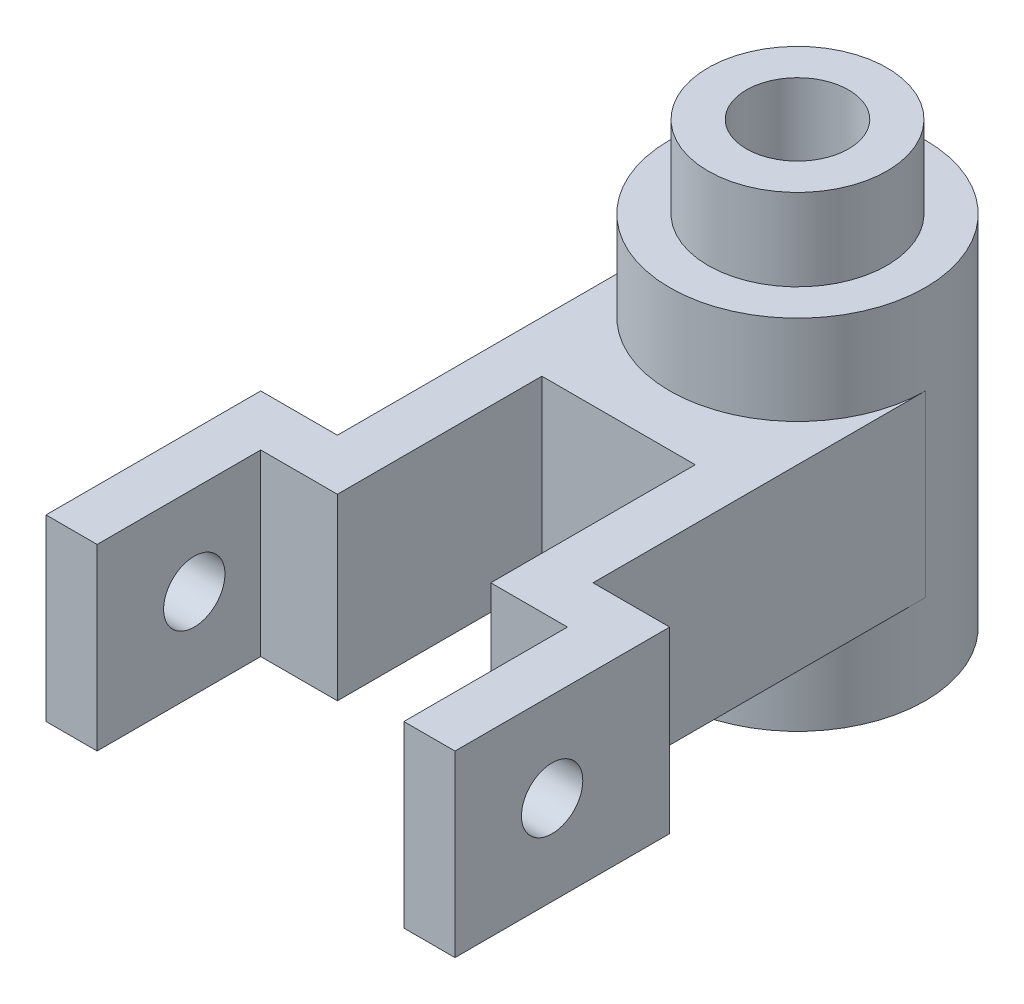
ISO-10303-21;
HEADER;
FILE_DESCRIPTION(('STEP AP214'),'2;1');
FILE_NAME('part.step','',(''),(''),'','','');
FILE_SCHEMA(('AUTOMOTIVE_DESIGN { 1 0 10303 214 1 1 1 1 }'));
ENDSEC;
DATA;
#1=APPLICATION_CONTEXT('core data for automotive mechanical design processes');
#2=APPLICATION_PROTOCOL_DEFINITION('international standard','automotive_design',2000,#1);
#3=PRODUCT_CONTEXT('',#1,'mechanical');
#4=PRODUCT('Part','Part','',(#3));
#5=PRODUCT_RELATED_PRODUCT_CATEGORY('part','',(#4));
#6=PRODUCT_DEFINITION_FORMATION('','',#4);
#7=PRODUCT_DEFINITION_CONTEXT('part definition',#1,'design');
#8=PRODUCT_DEFINITION('design','',#6,#7);
#9=PRODUCT_DEFINITION_SHAPE('','',#8);
#10=(LENGTH_UNIT() NAMED_UNIT(*) SI_UNIT(.MILLI.,.METRE.));
#11=(NAMED_UNIT(*) PLANE_ANGLE_UNIT() SI_UNIT($,.RADIAN.));
#12=(NAMED_UNIT(*) SI_UNIT($,.STERADIAN.) SOLID_ANGLE_UNIT());
#13=UNCERTAINTY_MEASURE_WITH_UNIT(LENGTH_MEASURE(1.E-05),#10,'distance_accuracy_value','');
#14=(GEOMETRIC_REPRESENTATION_CONTEXT(3) GLOBAL_UNCERTAINTY_ASSIGNED_CONTEXT((#13)) GLOBAL_UNIT_ASSIGNED_CONTEXT((#10,
#11,#12)) REPRESENTATION_CONTEXT('',''));
#15=CARTESIAN_POINT('',(0.,0.,0.));
#16=DIRECTION('',(0.,0.,1.));
#17=DIRECTION('',(1.,0.,0.));
#18=AXIS2_PLACEMENT_3D('',#15,#16,#17);
#19=CARTESIAN_POINT('',(0.,35.,0.));
#20=DIRECTION('',(0.,-1.,0.));
#21=DIRECTION('',(0.,0.,-1.));
#22=AXIS2_PLACEMENT_3D('',#19,#20,#21);
#23=CYLINDRICAL_SURFACE('',#22,25.);
#24=DIRECTION('',(0.,-1.,0.));
#25=VECTOR('',#24,1.);
#26=CARTESIAN_POINT('',(-25.,17.5,0.));
#27=LINE('',#26,#25);
#28=CARTESIAN_POINT('',(-25.,17.5,0.));
#29=VERTEX_POINT('',#28);
#30=CARTESIAN_POINT('',(-25.,-17.5,0.));
#31=VERTEX_POINT('',#30);
#32=EDGE_CURVE('E60',#29,#31,#27,.T.);
#33=ORIENTED_EDGE('',*,*,#32,.F.);
#34=CARTESIAN_POINT('',(0.,17.5,0.));
#35=DIRECTION('',(0.,1.,0.));
#36=DIRECTION('',(0.,0.,1.));
#37=AXIS2_PLACEMENT_3D('',#34,#35,#36);
#38=CIRCLE('',#37,25.);
#39=CARTESIAN_POINT('',(25.,17.5,0.));
#40=VERTEX_POINT('',#39);
#41=EDGE_CURVE('E65',#29,#40,#38,.T.);
#42=ORIENTED_EDGE('',*,*,#41,.T.);
#43=DIRECTION('',(0.,-1.,0.));
#44=VECTOR('',#43,1.);
#45=CARTESIAN_POINT('',(25.,17.5,0.));
#46=LINE('',#45,#44);
#47=CARTESIAN_POINT('',(25.,-17.5,0.));
#48=VERTEX_POINT('',#47);
#49=EDGE_CURVE('E205',#40,#48,#46,.T.);
#50=ORIENTED_EDGE('',*,*,#49,.T.);
#51=CARTESIAN_POINT('',(0.,-17.5,0.));
#52=DIRECTION('',(0.,1.,0.));
#53=DIRECTION('',(0.,0.,1.));
#54=AXIS2_PLACEMENT_3D('',#51,#52,#53);
#55=CIRCLE('',#54,25.);
#56=EDGE_CURVE('E207',#31,#48,#55,.T.);
#57=ORIENTED_EDGE('',*,*,#56,.F.);
#58=EDGE_LOOP('',(#33,#42,#50,#57));
#59=FACE_BOUND('',#58,.T.);
#60=CARTESIAN_POINT('',(0.,35.,0.));
#61=DIRECTION('',(0.,1.,0.));
#62=DIRECTION('',(0.,0.,1.));
#63=AXIS2_PLACEMENT_3D('',#60,#61,#62);
#64=CIRCLE('',#63,25.);
#65=CARTESIAN_POINT('',(0.,35.,25.));
#66=VERTEX_POINT('',#65);
#67=EDGE_CURVE('E11',#66,#66,#64,.T.);
#68=ORIENTED_EDGE('',*,*,#67,.F.);
#69=EDGE_LOOP('',(#68));
#70=FACE_BOUND('',#69,.T.);
#71=CARTESIAN_POINT('',(0.,-35.,0.));
#72=DIRECTION('',(0.,1.,0.));
#73=DIRECTION('',(0.,0.,1.));
#74=AXIS2_PLACEMENT_3D('',#71,#72,#73);
#75=CIRCLE('',#74,25.);
#76=CARTESIAN_POINT('',(0.,-35.,25.));
#77=VERTEX_POINT('',#76);
#78=EDGE_CURVE('E47',#77,#77,#75,.T.);
#79=ORIENTED_EDGE('',*,*,#78,.T.);
#80=EDGE_LOOP('',(#79));
#81=FACE_BOUND('',#80,.T.);
#82=ADVANCED_FACE('F41',(#59,#70,#81),#23,.T.);
#83=CARTESIAN_POINT('',(0.,35.,0.));
#84=DIRECTION('',(0.,1.,0.));
#85=DIRECTION('',(0.,0.,1.));
#86=AXIS2_PLACEMENT_3D('',#83,#84,#85);
#87=PLANE('',#86);
#88=CARTESIAN_POINT('',(0.,35.,0.));
#89=DIRECTION('',(0.,1.,0.));
#90=DIRECTION('',(0.,0.,1.));
#91=AXIS2_PLACEMENT_3D('',#88,#89,#90);
#92=CIRCLE('',#91,17.5);
#93=CARTESIAN_POINT('',(0.,35.,17.5));
#94=VERTEX_POINT('',#93);
#95=EDGE_CURVE('E282',#94,#94,#92,.F.);
#96=ORIENTED_EDGE('',*,*,#95,.T.);
#97=EDGE_LOOP('',(#96));
#98=FACE_BOUND('',#97,.T.);
#99=ORIENTED_EDGE('',*,*,#67,.T.);
#100=EDGE_LOOP('',(#99));
#101=FACE_BOUND('',#100,.T.);
#102=ADVANCED_FACE('F290',(#98,#101),#87,.T.);
#103=CARTESIAN_POINT('',(0.,-35.,0.));
#104=DIRECTION('',(0.,1.,0.));
#105=DIRECTION('',(0.,0.,1.));
#106=AXIS2_PLACEMENT_3D('',#103,#104,#105);
#107=PLANE('',#106);
#108=CARTESIAN_POINT('',(0.,-35.,0.));
#109=DIRECTION('',(0.,1.,0.));
#110=DIRECTION('',(0.,0.,1.));
#111=AXIS2_PLACEMENT_3D('',#108,#109,#110);
#112=CIRCLE('',#111,10.);
#113=CARTESIAN_POINT('',(0.,-35.,10.));
#114=VERTEX_POINT('',#113);
#115=EDGE_CURVE('E276',#114,#114,#112,.T.);
#116=ORIENTED_EDGE('',*,*,#115,.T.);
#117=EDGE_LOOP('',(#116));
#118=FACE_BOUND('',#117,.T.);
#119=ORIENTED_EDGE('',*,*,#78,.F.);
#120=EDGE_LOOP('',(#119));
#121=FACE_BOUND('',#120,.T.);
#122=ADVANCED_FACE('F300',(#118,#121),#107,.F.);
#123=CARTESIAN_POINT('',(0.,51.,0.));
#124=DIRECTION('',(0.,-1.,0.));
#125=DIRECTION('',(0.,0.,-1.));
#126=AXIS2_PLACEMENT_3D('',#123,#124,#125);
#127=CYLINDRICAL_SURFACE('',#126,17.5);
#128=ORIENTED_EDGE('',*,*,#95,.F.);
#129=EDGE_LOOP('',(#128));
#130=FACE_BOUND('',#129,.T.);
#131=CARTESIAN_POINT('',(0.,51.,0.));
#132=DIRECTION('',(0.,1.,0.));
#133=DIRECTION('',(0.,0.,1.));
#134=AXIS2_PLACEMENT_3D('',#131,#132,#133);
#135=CIRCLE('',#134,17.5);
#136=CARTESIAN_POINT('',(0.,51.,17.5));
#137=VERTEX_POINT('',#136);
#138=EDGE_CURVE('E285',#137,#137,#135,.T.);
#139=ORIENTED_EDGE('',*,*,#138,.F.);
#140=EDGE_LOOP('',(#139));
#141=FACE_BOUND('',#140,.T.);
#142=ADVANCED_FACE('F291',(#130,#141),#127,.T.);
#143=CARTESIAN_POINT('',(0.,51.,0.));
#144=DIRECTION('',(0.,1.,0.));
#145=DIRECTION('',(0.,0.,1.));
#146=AXIS2_PLACEMENT_3D('',#143,#144,#145);
#147=PLANE('',#146);
#148=CARTESIAN_POINT('',(0.,51.,0.));
#149=DIRECTION('',(0.,1.,0.));
#150=DIRECTION('',(0.,0.,1.));
#151=AXIS2_PLACEMENT_3D('',#148,#149,#150);
#152=CIRCLE('',#151,10.);
#153=CARTESIAN_POINT('',(0.,51.,10.));
#154=VERTEX_POINT('',#153);
#155=EDGE_CURVE('E42',#154,#154,#152,.T.);
#156=ORIENTED_EDGE('',*,*,#155,.F.);
#157=EDGE_LOOP('',(#156));
#158=FACE_BOUND('',#157,.T.);
#159=ORIENTED_EDGE('',*,*,#138,.T.);
#160=EDGE_LOOP('',(#159));
#161=FACE_BOUND('',#160,.T.);
#162=ADVANCED_FACE('F298',(#158,#161),#147,.T.);
#163=CARTESIAN_POINT('',(0.,-55.,0.));
#164=DIRECTION('',(0.,1.,0.));
#165=DIRECTION('',(0.,0.,1.));
#166=AXIS2_PLACEMENT_3D('',#163,#164,#165);
#167=CYLINDRICAL_SURFACE('',#166,10.);
#168=ORIENTED_EDGE('',*,*,#155,.T.);
#169=EDGE_LOOP('',(#168));
#170=FACE_BOUND('',#169,.T.);
#171=ORIENTED_EDGE('',*,*,#115,.F.);
#172=EDGE_LOOP('',(#171));
#173=FACE_BOUND('',#172,.T.);
#174=ADVANCED_FACE('F305',(#170,#173),#167,.F.);
#175=CARTESIAN_POINT('',(-25.,17.5,0.));
#176=DIRECTION('',(1.,0.,0.));
#177=DIRECTION('',(0.,0.,-1.));
#178=AXIS2_PLACEMENT_3D('',#175,#176,#177);
#179=PLANE('',#178);
#180=DIRECTION('',(0.,0.,1.));
#181=VECTOR('',#180,1.);
#182=CARTESIAN_POINT('',(-25.,-17.5,0.));
#183=LINE('',#182,#181);
#184=CARTESIAN_POINT('',(-25.,-17.5,65.));
#185=VERTEX_POINT('',#184);
#186=EDGE_CURVE('E164',#31,#185,#183,.T.);
#187=ORIENTED_EDGE('',*,*,#186,.T.);
#188=DIRECTION('',(0.,-1.,0.));
#189=VECTOR('',#188,1.);
#190=CARTESIAN_POINT('',(-25.,17.5,65.));
#191=LINE('',#190,#189);
#192=CARTESIAN_POINT('',(-25.,17.5,65.));
#193=VERTEX_POINT('',#192);
#194=EDGE_CURVE('E162',#193,#185,#191,.T.);
#195=ORIENTED_EDGE('',*,*,#194,.F.);
#196=DIRECTION('',(0.,0.,1.));
#197=VECTOR('',#196,1.);
#198=CARTESIAN_POINT('',(-25.,17.5,0.));
#199=LINE('',#198,#197);
#200=EDGE_CURVE('E155',#29,#193,#199,.T.);
#201=ORIENTED_EDGE('',*,*,#200,.F.);
#202=ORIENTED_EDGE('',*,*,#32,.T.);
#203=EDGE_LOOP('',(#187,#195,#201,#202));
#204=FACE_BOUND('',#203,.T.);
#205=ADVANCED_FACE('F161',(#204),#179,.F.);
#206=CARTESIAN_POINT('',(0.,17.5,65.));
#207=DIRECTION('',(0.,0.,1.));
#208=DIRECTION('',(1.,0.,0.));
#209=AXIS2_PLACEMENT_3D('',#206,#207,#208);
#210=PLANE('',#209);
#211=DIRECTION('',(-1.,0.,0.));
#212=VECTOR('',#211,1.);
#213=CARTESIAN_POINT('',(0.,-17.5,65.));
#214=LINE('',#213,#212);
#215=CARTESIAN_POINT('',(-40.,-17.5,65.));
#216=VERTEX_POINT('',#215);
#217=EDGE_CURVE('E212',#185,#216,#214,.T.);
#218=ORIENTED_EDGE('',*,*,#217,.T.);
#219=DIRECTION('',(0.,-1.,0.));
#220=VECTOR('',#219,1.);
#221=CARTESIAN_POINT('',(-40.,17.5,65.));
#222=LINE('',#221,#220);
#223=CARTESIAN_POINT('',(-40.,17.5,65.));
#224=VERTEX_POINT('',#223);
#225=EDGE_CURVE('E166',#224,#216,#222,.T.);
#226=ORIENTED_EDGE('',*,*,#225,.F.);
#227=DIRECTION('',(-1.,0.,0.));
#228=VECTOR('',#227,1.);
#229=CARTESIAN_POINT('',(0.,17.5,65.));
#230=LINE('',#229,#228);
#231=EDGE_CURVE('E156',#193,#224,#230,.T.);
#232=ORIENTED_EDGE('',*,*,#231,.F.);
#233=ORIENTED_EDGE('',*,*,#194,.T.);
#234=EDGE_LOOP('',(#218,#226,#232,#233));
#235=FACE_BOUND('',#234,.T.);
#236=ADVANCED_FACE('F167',(#235),#210,.F.);
#237=CARTESIAN_POINT('',(-40.,17.5,0.));
#238=DIRECTION('',(1.,0.,0.));
#239=DIRECTION('',(0.,0.,-1.));
#240=AXIS2_PLACEMENT_3D('',#237,#238,#239);
#241=PLANE('',#240);
#242=CARTESIAN_POINT('',(-40.,0.,88.));
#243=DIRECTION('',(1.,0.,0.));
#244=DIRECTION('',(0.,0.,-1.));
#245=AXIS2_PLACEMENT_3D('',#242,#243,#244);
#246=CIRCLE('',#245,6.);
#247=CARTESIAN_POINT('',(-40.,0.,82.));
#248=VERTEX_POINT('',#247);
#249=EDGE_CURVE('E209',#248,#248,#246,.T.);
#250=ORIENTED_EDGE('',*,*,#249,.T.);
#251=EDGE_LOOP('',(#250));
#252=FACE_BOUND('',#251,.T.);
#253=DIRECTION('',(0.,0.,1.));
#254=VECTOR('',#253,1.);
#255=CARTESIAN_POINT('',(-40.,-17.5,0.));
#256=LINE('',#255,#254);
#257=CARTESIAN_POINT('',(-40.,-17.5,107.));
#258=VERTEX_POINT('',#257);
#259=EDGE_CURVE('E214',#216,#258,#256,.T.);
#260=ORIENTED_EDGE('',*,*,#259,.T.);
#261=DIRECTION('',(0.,-1.,0.));
#262=VECTOR('',#261,1.);
#263=CARTESIAN_POINT('',(-40.,17.5,107.));
#264=LINE('',#263,#262);
#265=CARTESIAN_POINT('',(-40.,17.5,107.));
#266=VERTEX_POINT('',#265);
#267=EDGE_CURVE('E274',#266,#258,#264,.T.);
#268=ORIENTED_EDGE('',*,*,#267,.F.);
#269=DIRECTION('',(0.,0.,1.));
#270=VECTOR('',#269,1.);
#271=CARTESIAN_POINT('',(-40.,17.5,0.));
#272=LINE('',#271,#270);
#273=EDGE_CURVE('E173',#224,#266,#272,.T.);
#274=ORIENTED_EDGE('',*,*,#273,.F.);
#275=ORIENTED_EDGE('',*,*,#225,.T.);
#276=EDGE_LOOP('',(#260,#268,#274,#275));
#277=FACE_BOUND('',#276,.T.);
#278=ADVANCED_FACE('F368',(#252,#277),#241,.F.);
#279=CARTESIAN_POINT('',(0.,17.5,107.));
#280=DIRECTION('',(0.,0.,-1.));
#281=DIRECTION('',(-1.,0.,0.));
#282=AXIS2_PLACEMENT_3D('',#279,#280,#281);
#283=PLANE('',#282);
#284=DIRECTION('',(1.,0.,0.));
#285=VECTOR('',#284,1.);
#286=CARTESIAN_POINT('',(0.,-17.5,107.));
#287=LINE('',#286,#285);
#288=CARTESIAN_POINT('',(-30.,-17.5,107.));
#289=VERTEX_POINT('',#288);
#290=EDGE_CURVE('E213',#258,#289,#287,.T.);
#291=ORIENTED_EDGE('',*,*,#290,.T.);
#292=DIRECTION('',(0.,-1.,0.));
#293=VECTOR('',#292,1.);
#294=CARTESIAN_POINT('',(-30.,17.5,107.));
#295=LINE('',#294,#293);
#296=CARTESIAN_POINT('',(-30.,17.5,107.));
#297=VERTEX_POINT('',#296);
#298=EDGE_CURVE('E272',#297,#289,#295,.T.);
#299=ORIENTED_EDGE('',*,*,#298,.F.);
#300=DIRECTION('',(1.,0.,0.));
#301=VECTOR('',#300,1.);
#302=CARTESIAN_POINT('',(0.,17.5,107.));
#303=LINE('',#302,#301);
#304=EDGE_CURVE('E174',#266,#297,#303,.T.);
#305=ORIENTED_EDGE('',*,*,#304,.F.);
#306=ORIENTED_EDGE('',*,*,#267,.T.);
#307=EDGE_LOOP('',(#291,#299,#305,#306));
#308=FACE_BOUND('',#307,.T.);
#309=ADVANCED_FACE('F376',(#308),#283,.F.);
#310=CARTESIAN_POINT('',(-30.,17.5,0.));
#311=DIRECTION('',(-1.,0.,0.));
#312=DIRECTION('',(0.,0.,1.));
#313=AXIS2_PLACEMENT_3D('',#310,#311,#312);
#314=PLANE('',#313);
#315=CARTESIAN_POINT('',(-30.,0.,88.));
#316=DIRECTION('',(-1.,0.,0.));
#317=DIRECTION('',(0.,0.,1.));
#318=AXIS2_PLACEMENT_3D('',#315,#316,#317);
#319=CIRCLE('',#318,6.);
#320=CARTESIAN_POINT('',(-30.,0.,94.));
#321=VERTEX_POINT('',#320);
#322=EDGE_CURVE('E544',#321,#321,#319,.T.);
#323=ORIENTED_EDGE('',*,*,#322,.T.);
#324=EDGE_LOOP('',(#323));
#325=FACE_BOUND('',#324,.T.);
#326=DIRECTION('',(0.,0.,-1.));
#327=VECTOR('',#326,1.);
#328=CARTESIAN_POINT('',(-30.,-17.5,0.));
#329=LINE('',#328,#327);
#330=CARTESIAN_POINT('',(-30.,-17.5,75.));
#331=VERTEX_POINT('',#330);
#332=EDGE_CURVE('E220',#289,#331,#329,.T.);
#333=ORIENTED_EDGE('',*,*,#332,.T.);
#334=DIRECTION('',(0.,-1.,0.));
#335=VECTOR('',#334,1.);
#336=CARTESIAN_POINT('',(-30.,17.5,75.));
#337=LINE('',#336,#335);
#338=CARTESIAN_POINT('',(-30.,17.5,75.));
#339=VERTEX_POINT('',#338);
#340=EDGE_CURVE('E269',#339,#331,#337,.T.);
#341=ORIENTED_EDGE('',*,*,#340,.F.);
#342=DIRECTION('',(0.,0.,-1.));
#343=VECTOR('',#342,1.);
#344=CARTESIAN_POINT('',(-30.,17.5,0.));
#345=LINE('',#344,#343);
#346=EDGE_CURVE('E179',#297,#339,#345,.T.);
#347=ORIENTED_EDGE('',*,*,#346,.F.);
#348=ORIENTED_EDGE('',*,*,#298,.T.);
#349=EDGE_LOOP('',(#333,#341,#347,#348));
#350=FACE_BOUND('',#349,.T.);
#351=ADVANCED_FACE('F383',(#325,#350),#314,.F.);
#352=CARTESIAN_POINT('',(0.,17.5,75.));
#353=DIRECTION('',(0.,0.,-1.));
#354=DIRECTION('',(-1.,0.,0.));
#355=AXIS2_PLACEMENT_3D('',#352,#353,#354);
#356=PLANE('',#355);
#357=DIRECTION('',(1.,0.,0.));
#358=VECTOR('',#357,1.);
#359=CARTESIAN_POINT('',(0.,-17.5,75.));
#360=LINE('',#359,#358);
#361=CARTESIAN_POINT('',(-15.,-17.5,75.));
#362=VERTEX_POINT('',#361);
#363=EDGE_CURVE('E217',#331,#362,#360,.T.);
#364=ORIENTED_EDGE('',*,*,#363,.T.);
#365=DIRECTION('',(0.,-1.,0.));
#366=VECTOR('',#365,1.);
#367=CARTESIAN_POINT('',(-15.,17.5,75.));
#368=LINE('',#367,#366);
#369=CARTESIAN_POINT('',(-15.,17.5,75.));
#370=VERTEX_POINT('',#369);
#371=EDGE_CURVE('E264',#370,#362,#368,.T.);
#372=ORIENTED_EDGE('',*,*,#371,.F.);
#373=DIRECTION('',(1.,0.,0.));
#374=VECTOR('',#373,1.);
#375=CARTESIAN_POINT('',(0.,17.5,75.));
#376=LINE('',#375,#374);
#377=EDGE_CURVE('E185',#339,#370,#376,.T.);
#378=ORIENTED_EDGE('',*,*,#377,.F.);
#379=ORIENTED_EDGE('',*,*,#340,.T.);
#380=EDGE_LOOP('',(#364,#372,#378,#379));
#381=FACE_BOUND('',#380,.T.);
#382=ADVANCED_FACE('F392',(#381),#356,.F.);
#383=CARTESIAN_POINT('',(-15.,17.5,0.));
#384=DIRECTION('',(-1.,0.,0.));
#385=DIRECTION('',(0.,0.,1.));
#386=AXIS2_PLACEMENT_3D('',#383,#384,#385);
#387=PLANE('',#386);
#388=DIRECTION('',(0.,0.,-1.));
#389=VECTOR('',#388,1.);
#390=CARTESIAN_POINT('',(-15.,-17.5,0.));
#391=LINE('',#390,#389);
#392=CARTESIAN_POINT('',(-15.,-17.5,35.));
#393=VERTEX_POINT('',#392);
#394=EDGE_CURVE('E221',#362,#393,#391,.T.);
#395=ORIENTED_EDGE('',*,*,#394,.T.);
#396=DIRECTION('',(0.,-1.,0.));
#397=VECTOR('',#396,1.);
#398=CARTESIAN_POINT('',(-15.,17.5,35.));
#399=LINE('',#398,#397);
#400=CARTESIAN_POINT('',(-15.,17.5,35.));
#401=VERTEX_POINT('',#400);
#402=EDGE_CURVE('E265',#401,#393,#399,.T.);
#403=ORIENTED_EDGE('',*,*,#402,.F.);
#404=DIRECTION('',(0.,0.,-1.));
#405=VECTOR('',#404,1.);
#406=CARTESIAN_POINT('',(-15.,17.5,0.));
#407=LINE('',#406,#405);
#408=EDGE_CURVE('E183',#370,#401,#407,.T.);
#409=ORIENTED_EDGE('',*,*,#408,.F.);
#410=ORIENTED_EDGE('',*,*,#371,.T.);
#411=EDGE_LOOP('',(#395,#403,#409,#410));
#412=FACE_BOUND('',#411,.T.);
#413=ADVANCED_FACE('F401',(#412),#387,.F.);
#414=CARTESIAN_POINT('',(0.,17.5,35.));
#415=DIRECTION('',(0.,0.,-1.));
#416=DIRECTION('',(-1.,0.,0.));
#417=AXIS2_PLACEMENT_3D('',#414,#415,#416);
#418=PLANE('',#417);
#419=DIRECTION('',(1.,0.,0.));
#420=VECTOR('',#419,1.);
#421=CARTESIAN_POINT('',(0.,-17.5,35.));
#422=LINE('',#421,#420);
#423=CARTESIAN_POINT('',(15.,-17.5,35.));
#424=VERTEX_POINT('',#423);
#425=EDGE_CURVE('E224',#393,#424,#422,.T.);
#426=ORIENTED_EDGE('',*,*,#425,.T.);
#427=DIRECTION('',(0.,-1.,0.));
#428=VECTOR('',#427,1.);
#429=CARTESIAN_POINT('',(15.,17.5,35.));
#430=LINE('',#429,#428);
#431=CARTESIAN_POINT('',(15.,17.5,35.));
#432=VERTEX_POINT('',#431);
#433=EDGE_CURVE('E256',#432,#424,#430,.T.);
#434=ORIENTED_EDGE('',*,*,#433,.F.);
#435=DIRECTION('',(1.,0.,0.));
#436=VECTOR('',#435,1.);
#437=CARTESIAN_POINT('',(0.,17.5,35.));
#438=LINE('',#437,#436);
#439=EDGE_CURVE('E187',#401,#432,#438,.T.);
#440=ORIENTED_EDGE('',*,*,#439,.F.);
#441=ORIENTED_EDGE('',*,*,#402,.T.);
#442=EDGE_LOOP('',(#426,#434,#440,#441));
#443=FACE_BOUND('',#442,.T.);
#444=ADVANCED_FACE('F415',(#443),#418,.F.);
#445=CARTESIAN_POINT('',(15.,17.5,0.));
#446=DIRECTION('',(1.,0.,0.));
#447=DIRECTION('',(0.,0.,-1.));
#448=AXIS2_PLACEMENT_3D('',#445,#446,#447);
#449=PLANE('',#448);
#450=DIRECTION('',(0.,0.,1.));
#451=VECTOR('',#450,1.);
#452=CARTESIAN_POINT('',(15.,-17.5,0.));
#453=LINE('',#452,#451);
#454=CARTESIAN_POINT('',(15.,-17.5,75.));
#455=VERTEX_POINT('',#454);
#456=EDGE_CURVE('E225',#424,#455,#453,.T.);
#457=ORIENTED_EDGE('',*,*,#456,.T.);
#458=DIRECTION('',(0.,-1.,0.));
#459=VECTOR('',#458,1.);
#460=CARTESIAN_POINT('',(15.,17.5,75.));
#461=LINE('',#460,#459);
#462=CARTESIAN_POINT('',(15.,17.5,75.));
#463=VERTEX_POINT('',#462);
#464=EDGE_CURVE('E257',#463,#455,#461,.T.);
#465=ORIENTED_EDGE('',*,*,#464,.F.);
#466=DIRECTION('',(0.,0.,1.));
#467=VECTOR('',#466,1.);
#468=CARTESIAN_POINT('',(15.,17.5,0.));
#469=LINE('',#468,#467);
#470=EDGE_CURVE('E189',#432,#463,#469,.T.);
#471=ORIENTED_EDGE('',*,*,#470,.F.);
#472=ORIENTED_EDGE('',*,*,#433,.T.);
#473=EDGE_LOOP('',(#457,#465,#471,#472));
#474=FACE_BOUND('',#473,.T.);
#475=ADVANCED_FACE('F423',(#474),#449,.F.);
#476=CARTESIAN_POINT('',(0.,17.5,75.));
#477=DIRECTION('',(0.,0.,-1.));
#478=DIRECTION('',(-1.,0.,0.));
#479=AXIS2_PLACEMENT_3D('',#476,#477,#478);
#480=PLANE('',#479);
#481=DIRECTION('',(1.,0.,0.));
#482=VECTOR('',#481,1.);
#483=CARTESIAN_POINT('',(0.,-17.5,75.));
#484=LINE('',#483,#482);
#485=CARTESIAN_POINT('',(30.,-17.5,75.));
#486=VERTEX_POINT('',#485);
#487=EDGE_CURVE('E227',#455,#486,#484,.T.);
#488=ORIENTED_EDGE('',*,*,#487,.T.);
#489=DIRECTION('',(0.,-1.,0.));
#490=VECTOR('',#489,1.);
#491=CARTESIAN_POINT('',(30.,17.5,75.));
#492=LINE('',#491,#490);
#493=CARTESIAN_POINT('',(30.,17.5,75.));
#494=VERTEX_POINT('',#493);
#495=EDGE_CURVE('E254',#494,#486,#492,.T.);
#496=ORIENTED_EDGE('',*,*,#495,.F.);
#497=DIRECTION('',(1.,0.,0.));
#498=VECTOR('',#497,1.);
#499=CARTESIAN_POINT('',(0.,17.5,75.));
#500=LINE('',#499,#498);
#501=EDGE_CURVE('E188',#463,#494,#500,.T.);
#502=ORIENTED_EDGE('',*,*,#501,.F.);
#503=ORIENTED_EDGE('',*,*,#464,.T.);
#504=EDGE_LOOP('',(#488,#496,#502,#503));
#505=FACE_BOUND('',#504,.T.);
#506=ADVANCED_FACE('F427',(#505),#480,.F.);
#507=CARTESIAN_POINT('',(30.,17.5,0.));
#508=DIRECTION('',(1.,0.,0.));
#509=DIRECTION('',(0.,0.,-1.));
#510=AXIS2_PLACEMENT_3D('',#507,#508,#509);
#511=PLANE('',#510);
#512=CARTESIAN_POINT('',(30.,0.,88.));
#513=DIRECTION('',(1.,0.,0.));
#514=DIRECTION('',(0.,0.,-1.));
#515=AXIS2_PLACEMENT_3D('',#512,#513,#514);
#516=CIRCLE('',#515,6.);
#517=CARTESIAN_POINT('',(30.,0.,82.));
#518=VERTEX_POINT('',#517);
#519=EDGE_CURVE('E548',#518,#518,#516,.T.);
#520=ORIENTED_EDGE('',*,*,#519,.T.);
#521=EDGE_LOOP('',(#520));
#522=FACE_BOUND('',#521,.T.);
#523=DIRECTION('',(0.,0.,1.));
#524=VECTOR('',#523,1.);
#525=CARTESIAN_POINT('',(30.,-17.5,0.));
#526=LINE('',#525,#524);
#527=CARTESIAN_POINT('',(30.,-17.5,107.));
#528=VERTEX_POINT('',#527);
#529=EDGE_CURVE('E230',#486,#528,#526,.T.);
#530=ORIENTED_EDGE('',*,*,#529,.T.);
#531=DIRECTION('',(0.,-1.,0.));
#532=VECTOR('',#531,1.);
#533=CARTESIAN_POINT('',(30.,17.5,107.));
#534=LINE('',#533,#532);
#535=CARTESIAN_POINT('',(30.,17.5,107.));
#536=VERTEX_POINT('',#535);
#537=EDGE_CURVE('E249',#536,#528,#534,.T.);
#538=ORIENTED_EDGE('',*,*,#537,.F.);
#539=DIRECTION('',(0.,0.,1.));
#540=VECTOR('',#539,1.);
#541=CARTESIAN_POINT('',(30.,17.5,0.));
#542=LINE('',#541,#540);
#543=EDGE_CURVE('E195',#494,#536,#542,.T.);
#544=ORIENTED_EDGE('',*,*,#543,.F.);
#545=ORIENTED_EDGE('',*,*,#495,.T.);
#546=EDGE_LOOP('',(#530,#538,#544,#545));
#547=FACE_BOUND('',#546,.T.);
#548=ADVANCED_FACE('F439',(#522,#547),#511,.F.);
#549=CARTESIAN_POINT('',(0.,17.5,107.));
#550=DIRECTION('',(0.,0.,-1.));
#551=DIRECTION('',(-1.,0.,0.));
#552=AXIS2_PLACEMENT_3D('',#549,#550,#551);
#553=PLANE('',#552);
#554=DIRECTION('',(1.,0.,0.));
#555=VECTOR('',#554,1.);
#556=CARTESIAN_POINT('',(0.,-17.5,107.));
#557=LINE('',#556,#555);
#558=CARTESIAN_POINT('',(40.,-17.5,107.));
#559=VERTEX_POINT('',#558);
#560=EDGE_CURVE('E233',#528,#559,#557,.T.);
#561=ORIENTED_EDGE('',*,*,#560,.T.);
#562=DIRECTION('',(0.,-1.,0.));
#563=VECTOR('',#562,1.);
#564=CARTESIAN_POINT('',(40.,17.5,107.));
#565=LINE('',#564,#563);
#566=CARTESIAN_POINT('',(40.,17.5,107.));
#567=VERTEX_POINT('',#566);
#568=EDGE_CURVE('E247',#567,#559,#565,.T.);
#569=ORIENTED_EDGE('',*,*,#568,.F.);
#570=DIRECTION('',(1.,0.,0.));
#571=VECTOR('',#570,1.);
#572=CARTESIAN_POINT('',(0.,17.5,107.));
#573=LINE('',#572,#571);
#574=EDGE_CURVE('E191',#536,#567,#573,.T.);
#575=ORIENTED_EDGE('',*,*,#574,.F.);
#576=ORIENTED_EDGE('',*,*,#537,.T.);
#577=EDGE_LOOP('',(#561,#569,#575,#576));
#578=FACE_BOUND('',#577,.T.);
#579=ADVANCED_FACE('F446',(#578),#553,.F.);
#580=CARTESIAN_POINT('',(40.,17.5,0.));
#581=DIRECTION('',(1.,0.,0.));
#582=DIRECTION('',(0.,0.,-1.));
#583=AXIS2_PLACEMENT_3D('',#580,#581,#582);
#584=PLANE('',#583);
#585=CARTESIAN_POINT('',(40.,0.,88.));
#586=DIRECTION('',(1.,0.,0.));
#587=DIRECTION('',(0.,0.,-1.));
#588=AXIS2_PLACEMENT_3D('',#585,#586,#587);
#589=CIRCLE('',#588,6.);
#590=CARTESIAN_POINT('',(40.,0.,82.));
#591=VERTEX_POINT('',#590);
#592=EDGE_CURVE('E555',#591,#591,#589,.T.);
#593=ORIENTED_EDGE('',*,*,#592,.F.);
#594=EDGE_LOOP('',(#593));
#595=FACE_BOUND('',#594,.T.);
#596=DIRECTION('',(0.,0.,1.));
#597=VECTOR('',#596,1.);
#598=CARTESIAN_POINT('',(40.,-17.5,0.));
#599=LINE('',#598,#597);
#600=CARTESIAN_POINT('',(40.,-17.5,65.));
#601=VERTEX_POINT('',#600);
#602=EDGE_CURVE('E234',#601,#559,#599,.T.);
#603=ORIENTED_EDGE('',*,*,#602,.F.);
#604=DIRECTION('',(0.,-1.,0.));
#605=VECTOR('',#604,1.);
#606=CARTESIAN_POINT('',(40.,17.5,65.));
#607=LINE('',#606,#605);
#608=CARTESIAN_POINT('',(40.,17.5,65.));
#609=VERTEX_POINT('',#608);
#610=EDGE_CURVE('E246',#609,#601,#607,.T.);
#611=ORIENTED_EDGE('',*,*,#610,.F.);
#612=DIRECTION('',(0.,0.,1.));
#613=VECTOR('',#612,1.);
#614=CARTESIAN_POINT('',(40.,17.5,0.));
#615=LINE('',#614,#613);
#616=EDGE_CURVE('E196',#609,#567,#615,.T.);
#617=ORIENTED_EDGE('',*,*,#616,.T.);
#618=ORIENTED_EDGE('',*,*,#568,.T.);
#619=EDGE_LOOP('',(#603,#611,#617,#618));
#620=FACE_BOUND('',#619,.T.);
#621=ADVANCED_FACE('F458',(#595,#620),#584,.T.);
#622=CARTESIAN_POINT('',(0.,17.5,65.));
#623=DIRECTION('',(0.,0.,-1.));
#624=DIRECTION('',(-1.,0.,0.));
#625=AXIS2_PLACEMENT_3D('',#622,#623,#624);
#626=PLANE('',#625);
#627=DIRECTION('',(1.,0.,0.));
#628=VECTOR('',#627,1.);
#629=CARTESIAN_POINT('',(0.,-17.5,65.));
#630=LINE('',#629,#628);
#631=CARTESIAN_POINT('',(25.,-17.5,65.));
#632=VERTEX_POINT('',#631);
#633=EDGE_CURVE('E240',#632,#601,#630,.T.);
#634=ORIENTED_EDGE('',*,*,#633,.F.);
#635=DIRECTION('',(0.,-1.,0.));
#636=VECTOR('',#635,1.);
#637=CARTESIAN_POINT('',(25.,17.5,65.));
#638=LINE('',#637,#636);
#639=CARTESIAN_POINT('',(25.,17.5,65.));
#640=VERTEX_POINT('',#639);
#641=EDGE_CURVE('E242',#640,#632,#638,.T.);
#642=ORIENTED_EDGE('',*,*,#641,.F.);
#643=DIRECTION('',(1.,0.,0.));
#644=VECTOR('',#643,1.);
#645=CARTESIAN_POINT('',(0.,17.5,65.));
#646=LINE('',#645,#644);
#647=EDGE_CURVE('E197',#640,#609,#646,.T.);
#648=ORIENTED_EDGE('',*,*,#647,.T.);
#649=ORIENTED_EDGE('',*,*,#610,.T.);
#650=EDGE_LOOP('',(#634,#642,#648,#649));
#651=FACE_BOUND('',#650,.T.);
#652=ADVANCED_FACE('F470',(#651),#626,.T.);
#653=CARTESIAN_POINT('',(25.,17.5,0.));
#654=DIRECTION('',(1.,0.,0.));
#655=DIRECTION('',(0.,0.,-1.));
#656=AXIS2_PLACEMENT_3D('',#653,#654,#655);
#657=PLANE('',#656);
#658=DIRECTION('',(0.,0.,1.));
#659=VECTOR('',#658,1.);
#660=CARTESIAN_POINT('',(25.,-17.5,0.));
#661=LINE('',#660,#659);
#662=EDGE_CURVE('E239',#48,#632,#661,.T.);
#663=ORIENTED_EDGE('',*,*,#662,.F.);
#664=ORIENTED_EDGE('',*,*,#49,.F.);
#665=DIRECTION('',(0.,0.,1.));
#666=VECTOR('',#665,1.);
#667=CARTESIAN_POINT('',(25.,17.5,0.));
#668=LINE('',#667,#666);
#669=EDGE_CURVE('E202',#40,#640,#668,.T.);
#670=ORIENTED_EDGE('',*,*,#669,.T.);
#671=ORIENTED_EDGE('',*,*,#641,.T.);
#672=EDGE_LOOP('',(#663,#664,#670,#671));
#673=FACE_BOUND('',#672,.T.);
#674=ADVANCED_FACE('F476',(#673),#657,.T.);
#675=CARTESIAN_POINT('',(0.,17.5,0.));
#676=DIRECTION('',(0.,1.,0.));
#677=DIRECTION('',(0.,0.,1.));
#678=AXIS2_PLACEMENT_3D('',#675,#676,#677);
#679=PLANE('',#678);
#680=ORIENTED_EDGE('',*,*,#41,.F.);
#681=ORIENTED_EDGE('',*,*,#200,.T.);
#682=ORIENTED_EDGE('',*,*,#231,.T.);
#683=ORIENTED_EDGE('',*,*,#273,.T.);
#684=ORIENTED_EDGE('',*,*,#304,.T.);
#685=ORIENTED_EDGE('',*,*,#346,.T.);
#686=ORIENTED_EDGE('',*,*,#377,.T.);
#687=ORIENTED_EDGE('',*,*,#408,.T.);
#688=ORIENTED_EDGE('',*,*,#439,.T.);
#689=ORIENTED_EDGE('',*,*,#470,.T.);
#690=ORIENTED_EDGE('',*,*,#501,.T.);
#691=ORIENTED_EDGE('',*,*,#543,.T.);
#692=ORIENTED_EDGE('',*,*,#574,.T.);
#693=ORIENTED_EDGE('',*,*,#616,.F.);
#694=ORIENTED_EDGE('',*,*,#647,.F.);
#695=ORIENTED_EDGE('',*,*,#669,.F.);
#696=EDGE_LOOP('',(#680,#681,#682,#683,#684,#685,#686,#687,#688,#689,#690,#691,#692,#693,#694,#695));
#697=FACE_BOUND('',#696,.T.);
#698=ADVANCED_FACE('F152',(#697),#679,.T.);
#699=CARTESIAN_POINT('',(0.,-17.5,0.));
#700=DIRECTION('',(0.,1.,0.));
#701=DIRECTION('',(0.,0.,1.));
#702=AXIS2_PLACEMENT_3D('',#699,#700,#701);
#703=PLANE('',#702);
#704=ORIENTED_EDGE('',*,*,#56,.T.);
#705=ORIENTED_EDGE('',*,*,#662,.T.);
#706=ORIENTED_EDGE('',*,*,#633,.T.);
#707=ORIENTED_EDGE('',*,*,#602,.T.);
#708=ORIENTED_EDGE('',*,*,#560,.F.);
#709=ORIENTED_EDGE('',*,*,#529,.F.);
#710=ORIENTED_EDGE('',*,*,#487,.F.);
#711=ORIENTED_EDGE('',*,*,#456,.F.);
#712=ORIENTED_EDGE('',*,*,#425,.F.);
#713=ORIENTED_EDGE('',*,*,#394,.F.);
#714=ORIENTED_EDGE('',*,*,#363,.F.);
#715=ORIENTED_EDGE('',*,*,#332,.F.);
#716=ORIENTED_EDGE('',*,*,#290,.F.);
#717=ORIENTED_EDGE('',*,*,#259,.F.);
#718=ORIENTED_EDGE('',*,*,#217,.F.);
#719=ORIENTED_EDGE('',*,*,#186,.F.);
#720=EDGE_LOOP('',(#704,#705,#706,#707,#708,#709,#710,#711,#712,#713,#714,#715,#716,#717,#718,#719));
#721=FACE_BOUND('',#720,.T.);
#722=ADVANCED_FACE('F491',(#721),#703,.F.);
#723=CARTESIAN_POINT('',(-100.,0.,88.));
#724=DIRECTION('',(1.,0.,0.));
#725=DIRECTION('',(0.,0.,-1.));
#726=AXIS2_PLACEMENT_3D('',#723,#724,#725);
#727=CYLINDRICAL_SURFACE('',#726,6.);
#728=ORIENTED_EDGE('',*,*,#592,.T.);
#729=EDGE_LOOP('',(#728));
#730=FACE_BOUND('',#729,.T.);
#731=ORIENTED_EDGE('',*,*,#519,.F.);
#732=EDGE_LOOP('',(#731));
#733=FACE_BOUND('',#732,.T.);
#734=ADVANCED_FACE('F501',(#730,#733),#727,.F.);
#735=ORIENTED_EDGE('',*,*,#322,.F.);
#736=EDGE_LOOP('',(#735));
#737=FACE_BOUND('',#736,.T.);
#738=ORIENTED_EDGE('',*,*,#249,.F.);
#739=EDGE_LOOP('',(#738));
#740=FACE_BOUND('',#739,.T.);
#741=ADVANCED_FACE('F509',(#737,#740),#727,.F.);
#742=CLOSED_SHELL('',(#82,#102,#122,#142,#162,#174,#205,#236,#278,#309,#351,#382,#413,#444,#475,
#506,#548,#579,#621,#652,#674,#698,#722,#734,#741));
#743=MANIFOLD_SOLID_BREP('B2',#742);
#744=ADVANCED_BREP_SHAPE_REPRESENTATION('',(#18,#743),#14);
#745=SHAPE_DEFINITION_REPRESENTATION(#9,#744);
ENDSEC;
END-ISO-10303-21;
